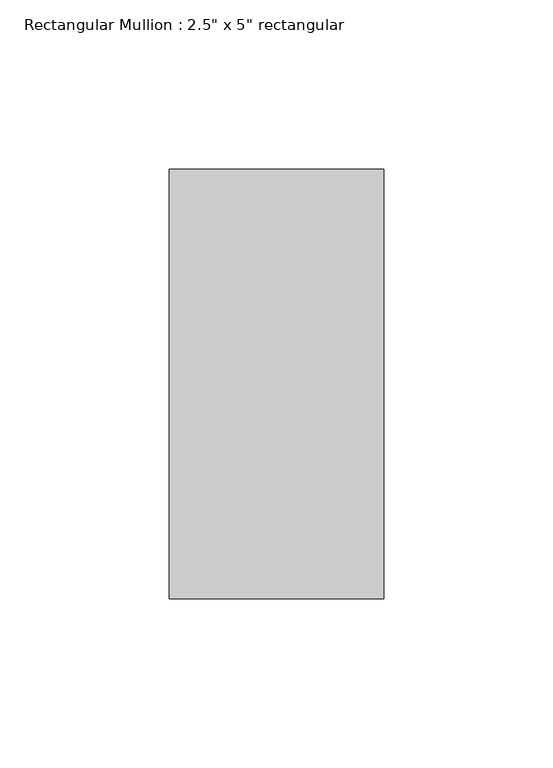
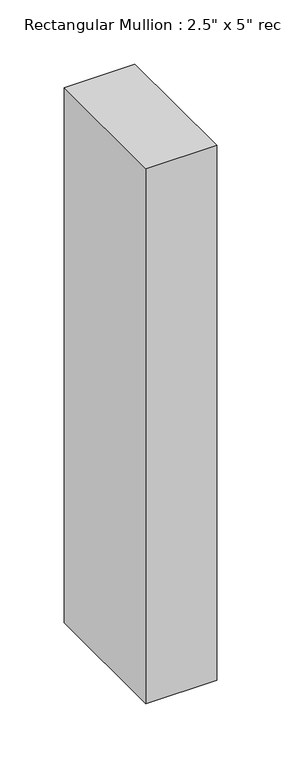
"""IFC4 building model written with IfcOpenShell, lengths in millimetres: member geometry."""

from ifc_helpers import new_model, si_unit, frame, origin, place, context, project, spatial, polyline, outline, extrude, source, transform, mapped, element, save


def member_7fd687a9(model_context):
    return source(origin(), model_context, "Body", "SweptSolid", [
        extrude(outline(polyline([(0.0, 63.5), (0.0, -63.5), (-63.5, -63.5), (-63.5, 63.5), (0.0, 63.5)])), frame((0.0, 0.0, -508.0), z_axis=(0.0, 0.0, 1.0), x_axis=(1.0, 0.0, 0.0)), (0.0, 0.0, 1.0), 508.0),
    ])


if __name__ == "__main__":
    model = new_model("IFC4")
    model_context = context("Model", 3, world=origin())
    ifc_project = project(units=[si_unit("LENGTHUNIT", "METRE", prefix="MILLI")], contexts=[model_context])
    site = spatial("IfcSite", under=ifc_project)
    building = spatial("IfcBuilding", under=site)
    placement = place(None, origin())
    member_shape = member_7fd687a9(model_context)
    element("IfcMember", 1, ObjectType="Rectangular Mullion : 2.5\" x 5\" rectangular", at=placement, inside=building, context=model_context, shape_type="MappedRepresentation", body=[
        mapped(member_shape, transform((0.0, 0.0, 0.0), x_axis=(1.0, 0.0, 0.0), y_axis=(0.0, 1.0, 0.0), z_axis=(0.0, 0.0, 1.0))),
    ])
    save(model, "model.ifc")

# Revit data of these elements
# Type "Rectangular Mullion : 2.5\" x 5\" rectangular"
#   built-in parameter 1007304 = 0.416667 (stored number, unit not read)
#   built-in parameter 1007301 = 0.104167 (stored number, unit not read)
#   built-in parameter 1007300 = 0.104167 (stored number, unit not read)
# Element 1 (IfcMember, "Rectangular Mullion : 2.5\" x 5\" rectangular")
#   Materials on its faces: "door colour"
# Materials
#   "door colour": class "Generic", colour RGB 120 120 120, transparency 0, Cost = 0
